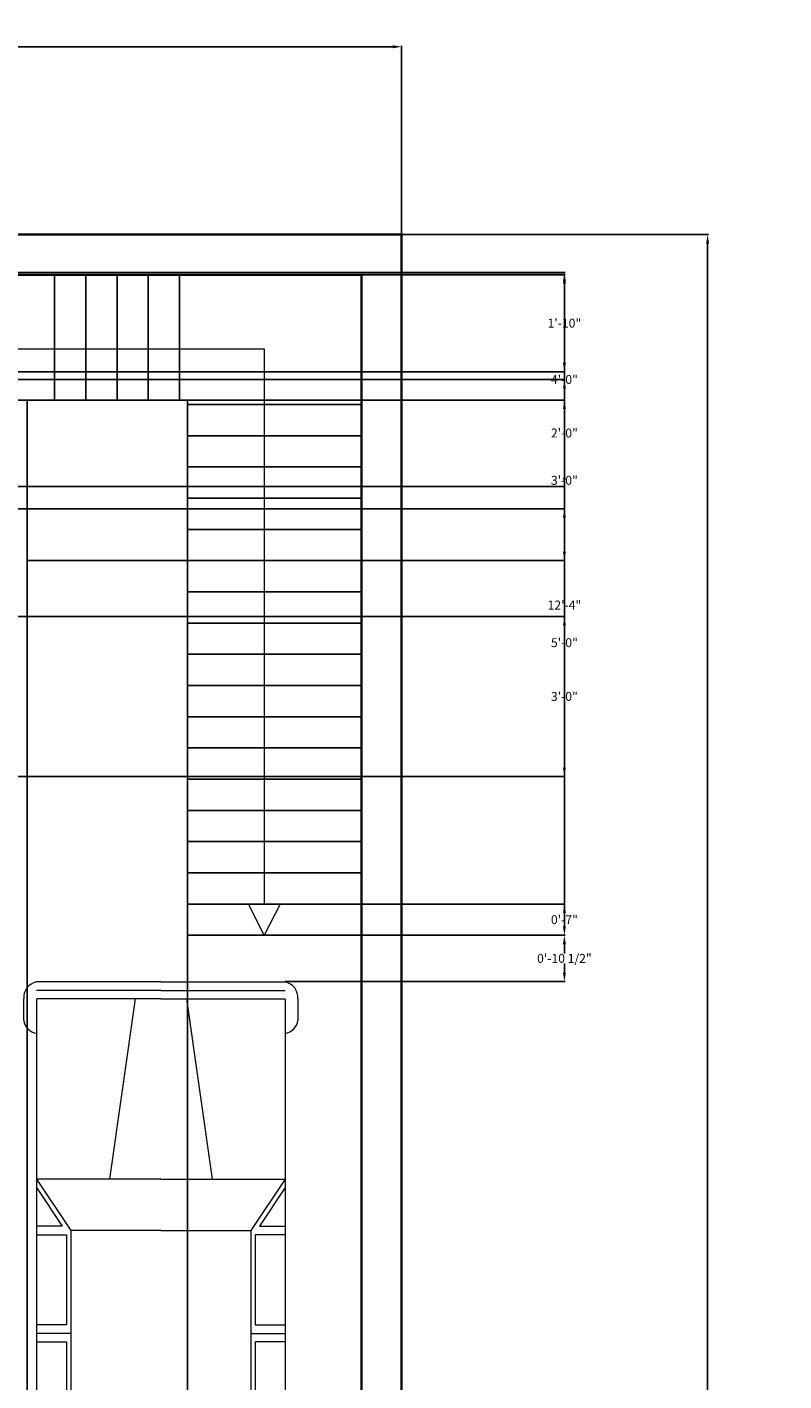
# Model space of a CAD drawing. Units: inches. Extents: x -83 to 408, y 158 to 919.
# Tile 5 of 5: x 238 to 408, y 586 to 889. Entities that reach past the tile are written whole.
import ezdxf

# ---------------------------------------------------------------- set-up
doc = ezdxf.new("R2010")
doc.units = ezdxf.units.IN
doc.header["$MEASUREMENT"] = 0
for name, color, linetype, lineweight in [('A-ANNO-DIMS', 2, 'Continuous', 18), ('A-ANNO-SYMB', 3, 'Continuous', 18), ('A-FLOR-STRS', 7, 'Continuous', 25), ('C-PKNG-VEHI', 8, 'Continuous', 18), ('L-WALL', 7, 'Continuous', 35)]:
    doc.layers.add(name, color=color, linetype=linetype, lineweight=lineweight)
doc.styles.get("Standard").update_dxf_attribs({"font": 'arial.ttf'})
doc.dimstyles.get("Standard").update_dxf_attribs({"dimtxt": 2, "dimasz": 2, "dimexe": 0.18, "dimexo": 0.0625, "dimgap": 0.09, "dimtad": 0, "dimtih": 1, "dimtoh": 1, "dimdec": 0, "dimzin": 0, "dimdsep": 46, "dimlunit": 3, "dimtxsty": 'Standard', "dimcen": 0.09, "dimadec": 0, "dimazin": 0, "dimtfac": 1, "dimtdec": 0, "dimtofl": 0, "dimtmove": 0, "dimatfit": 3, "dimfxl": 1, "dimtolj": 1, "dimtzin": 0, "dimarcsym": 0})

# ---------------------------------------------------------------- blocks, each defined once
blk = doc.blocks.new('*U15')
for p, q in [((5.44, 42.31), (12.12, 42.31)), ((189.69, 42.31), (183.01, 42.31)), ((0.1, -0.41), (0.1, 38.35)), ((2.77, -0.41), (2.77, 38.31)), ((5.44, -0.41), (5.44, 38.24)), ((5.45, 38.31), (16.12, 38.31)), ((16.12, 38.31), (180.34, 38.31)), ((61.52, -0.41), (61.52, 38.31)), ((61.52, 38.31), (77.54, 27.62)), ((64.19, 38.31), (76.2, 30.29)), ((76.2, 30.29), (76.2, 38.31)), ((78.87, 38.31), (78.87, 28.96)), ((106.91, 28.96), (106.91, 38.31)), ((109.58, 27.62), (109.58, 38.31)), ((112.25, 38.31), (112.25, 28.96)), ((140.29, 28.96), (140.29, 38.31)), ((141.62, 27.62), (149.64, 38.31)), ((149.64, -0.41), (149.64, 38.31)), ((189.69, 38.31), (179.01, 38.31)), ((189.69, -0.41), (189.69, 38.24)), ((192.36, -0.41), (192.36, 38.31)), ((195.03, -0.41), (195.03, 38.35)), ((77.54, 27.62), (141.62, 27.62)), ((77.54, -0.41), (77.54, 27.62)), ((78.87, 28.96), (106.91, 28.96)), ((112.25, 28.96), (140.29, 28.96)), ((141.62, -0.41), (141.62, 27.62)), ((5.44, 7.6), (61.52, 15.61)), ((0.1, -0.42), (0.1, -39.18)), ((2.77, -0.41), (2.77, -39.13)), ((5.44, -0.42), (5.44, -39.07)), ((61.52, -0.41), (61.52, -39.13)), ((77.54, -0.41), (77.54, -28.45)), ((141.62, -0.41), (141.62, -28.45)), ((149.64, -0.41), (149.64, -39.13)), ((189.69, -0.42), (189.69, -39.07)), ((192.36, -0.41), (192.36, -39.13)), ((195.03, -0.42), (195.03, -39.18)), ((5.44, -8.42), (61.52, -16.43)), ((61.52, -39.13), (77.54, -28.45)), ((77.54, -28.45), (141.62, -28.45)), ((109.58, -28.45), (109.58, -39.13)), ((141.62, -28.45), (149.64, -39.13)), ((64.19, -39.13), (76.2, -31.12)), ((76.2, -31.12), (76.2, -39.13)), ((78.87, -39.13), (78.87, -29.79)), ((78.87, -29.79), (106.91, -29.79)), ((106.91, -29.79), (106.91, -39.13)), ((112.25, -29.79), (140.29, -29.79)), ((112.25, -39.13), (112.25, -29.79)), ((140.29, -29.79), (140.29, -39.13)), ((5.45, -39.13), (16.12, -39.13)), ((16.12, -39.13), (180.34, -39.13)), ((189.69, -39.13), (179.01, -39.13)), ((5.44, -43.14), (12.12, -43.14)), ((189.69, -43.14), (183.01, -43.14))]:
    blk.add_line(p, q)
for centre, radius, start, end in [((5.06, 37.26), 5.06, 85.6455, 168.0943), ((11.45, 37.64), 4.72, 8.1301, 81.87), ((183.68, 37.64), 4.72, 98.13, 171.8699), ((190.07, 37.26), 5.06, 11.9057, 94.3545), ((5.06, -38.09), 5.06, 191.9057, 274.3545), ((11.45, -38.46), 4.72, 278.13, 351.8699), ((183.68, -38.46), 4.72, 188.1301, 261.87), ((190.07, -38.09), 5.06, 265.6455, 348.0943)]:
    blk.add_arc(centre, radius, start, end)
blk = doc.blocks.new('*D17')
at = {"layer": 'A-ANNO-DIMS', "color": 0, "lineweight": -2, "transparency": 16777216}
for p, q in [((322.25, 842.67), (390.98, 842.67)), ((390.8, 840.67), (390.8, 524.09)), ((390.8, 199.15), (390.8, 515.73)), ((322.25, 197.15), (390.98, 197.15))]:
    blk.add_line(p, q, dxfattribs=at)
at = {"layer": 'A-ANNO-DIMS', "color": 0, "transparency": 16777216}
for points in [[(390.47, 840.67), (391.14, 840.67), (390.8, 842.67)], [(390.47, 199.15), (391.14, 199.15), (390.8, 197.15)]]:
    blk.add_solid(points, dxfattribs=at)
at = {"layer": 'Defpoints', "color": 0, "transparency": 16777216}
for p in [(322.19, 842.67), (322.19, 197.15), (390.8, 197.15)]:
    blk.add_point(p, dxfattribs=at)
at = {"layer": 'A-ANNO-DIMS', "color": 0, "transparency": 16777216, "insert": (390.8, 519.91), "char_height": 2, "attachment_point": 5}
blk.add_mtext('\\A1;{\\H4x;53\'-10"}', dxfattribs=at)
blk = doc.blocks.new('*D18')
at = {"layer": 'A-ANNO-DIMS', "color": 0, "lineweight": -2, "transparency": 16777216}
for p, q in [((-40.81, 843.26), (-40.81, 884.97)), ((-38.81, 884.79), (126.86, 884.79)), ((320.19, 884.79), (154.52, 884.79)), ((322.19, 842.73), (322.19, 884.97))]:
    blk.add_line(p, q, dxfattribs=at)
at = {"layer": 'A-ANNO-DIMS', "color": 0, "transparency": 16777216}
for points in [[(-38.81, 885.12), (-38.81, 884.46), (-40.81, 884.79)], [(320.19, 885.12), (320.19, 884.46), (322.19, 884.79)]]:
    blk.add_solid(points, dxfattribs=at)
at = {"layer": 'Defpoints', "color": 0, "transparency": 16777216}
for p in [(322.19, 884.79), (-40.81, 843.2), (322.19, 842.67)]:
    blk.add_point(p, dxfattribs=at)
at = {"layer": 'A-ANNO-DIMS', "color": 0, "transparency": 16777216, "insert": (140.69, 884.79), "char_height": 2, "attachment_point": 5}
blk.add_mtext('\\A1;{\\H4x;30\'-3"}', dxfattribs=at)
blk = doc.blocks.new('*D48')
at = {"layer": 'A-ANNO-DIMS', "color": 0, "lineweight": -2, "transparency": 16777216}
for p, q in [((47.25, 834.2), (358.87, 834.2)), ((358.69, 832.2), (358.69, 811.31)), ((358.69, 788.2), (358.69, 809.09)), ((47.25, 786.2), (358.87, 786.2))]:
    blk.add_line(p, q, dxfattribs=at)
at = {"layer": 'A-ANNO-DIMS', "color": 0, "transparency": 16777216}
for points in [[(358.36, 832.2), (359.02, 832.2), (358.69, 834.2)], [(358.36, 788.2), (359.02, 788.2), (358.69, 786.2)]]:
    blk.add_solid(points, dxfattribs=at)
at = {"layer": 'Defpoints', "color": 0, "transparency": 16777216}
for p in [(47.19, 834.2), (47.19, 786.2), (358.69, 786.2)]:
    blk.add_point(p, dxfattribs=at)
at = {"layer": 'A-ANNO-DIMS', "color": 0, "transparency": 16777216, "insert": (358.69, 810.2), "char_height": 2, "attachment_point": 5}
blk.add_mtext('\\A1;4\'-0"', dxfattribs=at)
blk = doc.blocks.new('*D49')
at = {"layer": 'A-ANNO-DIMS', "color": 0, "lineweight": -2, "transparency": 16777216}
for p, q in [((47.25, 810.2), (358.87, 810.2)), ((358.69, 808.2), (358.69, 799.31)), ((358.69, 788.2), (358.69, 797.09)), ((47.25, 786.2), (358.87, 786.2))]:
    blk.add_line(p, q, dxfattribs=at)
at = {"layer": 'A-ANNO-DIMS', "color": 0, "transparency": 16777216}
for points in [[(358.36, 808.2), (359.02, 808.2), (358.69, 810.2)], [(358.36, 788.2), (359.02, 788.2), (358.69, 786.2)]]:
    blk.add_solid(points, dxfattribs=at)
at = {"layer": 'Defpoints', "color": 0, "transparency": 16777216}
for p in [(47.19, 810.2), (47.19, 786.2), (358.69, 786.2)]:
    blk.add_point(p, dxfattribs=at)
at = {"layer": 'A-ANNO-DIMS', "color": 0, "transparency": 16777216, "insert": (358.69, 798.2), "char_height": 2, "attachment_point": 5}
blk.add_mtext('\\A1;2\'-0"', dxfattribs=at)
blk = doc.blocks.new('*D50')
at = {"layer": 'A-ANNO-DIMS', "color": 0, "lineweight": -2, "transparency": 16777216}
for p, q in [((193.25, 757.08), (358.87, 757.08)), ((358.69, 755.08), (358.69, 740.25)), ((358.69, 723.2), (358.69, 738.03)), ((193.25, 721.2), (358.87, 721.2))]:
    blk.add_line(p, q, dxfattribs=at)
at = {"layer": 'A-ANNO-DIMS', "color": 0, "transparency": 16777216}
for points in [[(358.36, 755.08), (359.02, 755.08), (358.69, 757.08)], [(358.36, 723.2), (359.02, 723.2), (358.69, 721.2)]]:
    blk.add_solid(points, dxfattribs=at)
at = {"layer": 'Defpoints', "color": 0, "transparency": 16777216}
for p in [(193.19, 757.08), (193.19, 721.2), (358.69, 721.2)]:
    blk.add_point(p, dxfattribs=at)
at = {"layer": 'A-ANNO-DIMS', "color": 0, "transparency": 16777216, "insert": (358.69, 739.14), "char_height": 2, "attachment_point": 5}
blk.add_mtext('\\A1;3\'-0"', dxfattribs=at)
blk = doc.blocks.new('*D54')
at = {"layer": 'A-ANNO-DIMS', "color": 0, "lineweight": -2, "transparency": 16777216}
for p, q in [((193.25, 833.7), (358.87, 833.7)), ((358.69, 831.7), (358.69, 823.94)), ((358.69, 813.95), (358.69, 821.71)), ((193.25, 811.95), (358.87, 811.95))]:
    blk.add_line(p, q, dxfattribs=at)
at = {"layer": 'A-ANNO-DIMS', "color": 0, "transparency": 16777216}
for points in [[(358.36, 831.7), (359.02, 831.7), (358.69, 833.7)], [(358.36, 813.95), (359.02, 813.95), (358.69, 811.95)]]:
    blk.add_solid(points, dxfattribs=at)
at = {"layer": 'Defpoints', "color": 0, "transparency": 16777216}
for p in [(193.19, 833.7), (193.19, 811.95), (358.69, 811.95)]:
    blk.add_point(p, dxfattribs=at)
at = {"layer": 'A-ANNO-DIMS', "color": 0, "transparency": 16777216, "insert": (358.69, 822.83), "char_height": 2, "attachment_point": 5}
blk.add_mtext('\\A1;1\'-10"', dxfattribs=at)
blk = doc.blocks.new('*D56')
at = {"layer": 'A-ANNO-DIMS', "color": 0, "lineweight": -2, "transparency": 16777216}
for p, q in [((52.25, 781.2), (358.87, 781.2)), ((358.69, 779.2), (358.69, 752.31)), ((358.69, 723.2), (358.69, 750.09)), ((47.25, 721.2), (358.87, 721.2))]:
    blk.add_line(p, q, dxfattribs=at)
at = {"layer": 'A-ANNO-DIMS', "color": 0, "transparency": 16777216}
for points in [[(358.36, 779.2), (359.02, 779.2), (358.69, 781.2)], [(358.36, 723.2), (359.02, 723.2), (358.69, 721.2)]]:
    blk.add_solid(points, dxfattribs=at)
at = {"layer": 'Defpoints', "color": 0, "transparency": 16777216}
for p in [(52.19, 781.2), (47.19, 721.2), (358.69, 721.2)]:
    blk.add_point(p, dxfattribs=at)
at = {"layer": 'A-ANNO-DIMS', "color": 0, "transparency": 16777216, "insert": (358.69, 751.2), "char_height": 2, "attachment_point": 5}
blk.add_mtext('\\A1;5\'-0"', dxfattribs=at)
blk = doc.blocks.new('*D57')
at = {"layer": 'A-ANNO-DIMS', "color": 0, "lineweight": -2, "transparency": 16777216}
for p, q in [((274.19, 685.53), (274.19, 160.47)), ((313.19, 685.53), (313.19, 160.47)), ((276.19, 160.65), (290.94, 160.65)), ((311.19, 160.65), (296.44, 160.65))]:
    blk.add_line(p, q, dxfattribs=at)
at = {"layer": 'A-ANNO-DIMS', "color": 0, "transparency": 16777216}
for points in [[(276.19, 160.98), (276.19, 160.32), (274.19, 160.65)], [(311.19, 160.98), (311.19, 160.32), (313.19, 160.65)]]:
    blk.add_solid(points, dxfattribs=at)
at = {"layer": 'Defpoints', "color": 0, "transparency": 16777216}
for p in [(274.19, 685.59), (313.19, 685.59), (313.19, 160.65)]:
    blk.add_point(p, dxfattribs=at)
at = {"layer": 'A-ANNO-DIMS', "color": 0, "transparency": 16777216, "insert": (293.69, 160.65), "char_height": 2, "attachment_point": 5}
blk.add_mtext('\\A1;3\'-3"', dxfattribs=at)
blk = doc.blocks.new('*D58')
at = {"layer": 'A-ANNO-DIMS', "color": 0, "lineweight": -2, "transparency": 16777216}
for p, q in [((313.25, 833.67), (358.87, 833.67)), ((358.69, 831.67), (358.69, 760.72)), ((358.69, 687.59), (358.69, 758.54)), ((313.25, 685.59), (358.87, 685.59))]:
    blk.add_line(p, q, dxfattribs=at)
at = {"layer": 'A-ANNO-DIMS', "color": 0, "transparency": 16777216}
for points in [[(358.36, 831.67), (359.02, 831.67), (358.69, 833.67)], [(358.36, 687.59), (359.02, 687.59), (358.69, 685.59)]]:
    blk.add_solid(points, dxfattribs=at)
at = {"layer": 'Defpoints', "color": 0, "transparency": 16777216}
for p in [(313.19, 833.67), (358.69, 833.67), (313.19, 685.59)]:
    blk.add_point(p, dxfattribs=at)
at = {"layer": 'A-ANNO-DIMS', "color": 0, "transparency": 16777216, "insert": (358.69, 759.63), "char_height": 2, "attachment_point": 5}
blk.add_mtext('\\A1;12\'-4"', dxfattribs=at)
blk = doc.blocks.new('*D59')
at = {"layer": 'A-ANNO-DIMS', "color": 0, "lineweight": -2, "transparency": 16777216}
for p, q in [((202.19, 769.53), (202.19, 160.47)), ((238.19, 769.53), (238.19, 160.47)), ((204.19, 160.65), (217.44, 160.65)), ((236.19, 160.65), (222.94, 160.65))]:
    blk.add_line(p, q, dxfattribs=at)
at = {"layer": 'A-ANNO-DIMS', "color": 0, "transparency": 16777216}
for points in [[(204.19, 160.98), (204.19, 160.32), (202.19, 160.65)], [(236.19, 160.98), (236.19, 160.32), (238.19, 160.65)]]:
    blk.add_solid(points, dxfattribs=at)
at = {"layer": 'Defpoints', "color": 0, "transparency": 16777216}
for p in [(202.19, 769.59), (238.19, 769.59), (238.19, 160.65)]:
    blk.add_point(p, dxfattribs=at)
at = {"layer": 'A-ANNO-DIMS', "color": 0, "transparency": 16777216, "insert": (220.19, 160.65), "char_height": 2, "attachment_point": 5}
blk.add_mtext('\\A1;3\'-0"', dxfattribs=at)
blk = doc.blocks.new('*D60')
at = {"layer": 'A-ANNO-DIMS', "color": 0, "lineweight": -2, "transparency": 16777216}
for p, q in [((238.19, 805.53), (238.19, 160.47)), ((274.19, 805.53), (274.19, 160.47)), ((240.19, 160.65), (253.44, 160.65)), ((272.19, 160.65), (258.94, 160.65))]:
    blk.add_line(p, q, dxfattribs=at)
at = {"layer": 'A-ANNO-DIMS', "color": 0, "transparency": 16777216}
for points in [[(240.19, 160.98), (240.19, 160.32), (238.19, 160.65)], [(272.19, 160.98), (272.19, 160.32), (274.19, 160.65)]]:
    blk.add_solid(points, dxfattribs=at)
at = {"layer": 'Defpoints', "color": 0, "transparency": 16777216}
for p in [(238.19, 805.59), (274.19, 805.59), (274.19, 160.65)]:
    blk.add_point(p, dxfattribs=at)
at = {"layer": 'A-ANNO-DIMS', "color": 0, "transparency": 16777216, "insert": (256.19, 160.65), "char_height": 2, "attachment_point": 5}
blk.add_mtext('\\A1;3\'-0"', dxfattribs=at)
blk = doc.blocks.new('*D61')
at = {"layer": 'A-ANNO-DIMS', "color": 0, "lineweight": -2, "transparency": 16777216}
for p, q in [((238.25, 805.59), (358.87, 805.59)), ((358.69, 803.59), (358.69, 788.71)), ((358.69, 771.59), (358.69, 786.48)), ((238.25, 769.59), (358.87, 769.59))]:
    blk.add_line(p, q, dxfattribs=at)
at = {"layer": 'A-ANNO-DIMS', "color": 0, "transparency": 16777216}
for points in [[(358.36, 803.59), (359.02, 803.59), (358.69, 805.59)], [(358.36, 771.59), (359.02, 771.59), (358.69, 769.59)]]:
    blk.add_solid(points, dxfattribs=at)
at = {"layer": 'Defpoints', "color": 0, "transparency": 16777216}
for p in [(238.19, 805.59), (358.69, 805.59), (238.19, 769.59)]:
    blk.add_point(p, dxfattribs=at)
at = {"layer": 'A-ANNO-DIMS', "color": 0, "transparency": 16777216, "insert": (358.69, 787.59), "char_height": 2, "attachment_point": 5}
blk.add_mtext('\\A1;3\'-0"', dxfattribs=at)
blk = doc.blocks.new('*D62')
at = {"layer": 'A-ANNO-DIMS', "color": 0, "lineweight": -2, "transparency": 16777216}
for p, q in [((272.31, 833.67), (-77.49, 833.67)), ((-77.31, 831.67), (-77.31, 820.72)), ((-77.31, 807.59), (-77.31, 818.54)), ((274.13, 805.59), (-77.49, 805.59))]:
    blk.add_line(p, q, dxfattribs=at)
at = {"layer": 'A-ANNO-DIMS', "color": 0, "transparency": 16777216}
for points in [[(-77.64, 831.67), (-76.98, 831.67), (-77.31, 833.67)], [(-77.64, 807.59), (-76.98, 807.59), (-77.31, 805.59)]]:
    blk.add_solid(points, dxfattribs=at)
at = {"layer": 'Defpoints', "color": 0, "transparency": 16777216}
for p in [(-77.31, 833.67), (272.37, 833.67), (274.19, 805.59)]:
    blk.add_point(p, dxfattribs=at)
at = {"layer": 'A-ANNO-DIMS', "color": 0, "transparency": 16777216, "insert": (-77.31, 819.63), "char_height": 2, "attachment_point": 5}
blk.add_mtext('\\A1;2\'-4"', dxfattribs=at)
blk = doc.blocks.new('*D63')
at = {"layer": 'A-ANNO-DIMS', "color": 0, "lineweight": -2, "transparency": 16777216}
for p, q in [((313.25, 692.59), (358.87, 692.59)), ((358.69, 690.59), (358.69, 690.2)), ((358.69, 687.59), (358.69, 687.98)), ((313.25, 685.59), (358.87, 685.59))]:
    blk.add_line(p, q, dxfattribs=at)
at = {"layer": 'A-ANNO-DIMS', "color": 0, "transparency": 16777216}
for points in [[(358.36, 690.59), (359.02, 690.59), (358.69, 692.59)], [(358.36, 687.59), (359.02, 687.59), (358.69, 685.59)]]:
    blk.add_solid(points, dxfattribs=at)
at = {"layer": 'Defpoints', "color": 0, "transparency": 16777216}
for p in [(313.19, 692.59), (358.69, 692.59), (313.19, 685.59)]:
    blk.add_point(p, dxfattribs=at)
at = {"layer": 'A-ANNO-DIMS', "color": 0, "transparency": 16777216, "insert": (358.69, 689.09), "char_height": 2, "attachment_point": 5}
blk.add_mtext('\\A1;0\'-7"', dxfattribs=at)
blk = doc.blocks.new('*D70')
at = {"layer": 'A-ANNO-DIMS', "color": 0, "lineweight": -2, "transparency": 16777216}
for p, q in [((313.25, 685.59), (358.87, 685.59)), ((358.69, 683.59), (358.69, 681.54)), ((358.69, 677.24), (358.69, 679.29)), ((296.03, 675.24), (358.87, 675.24))]:
    blk.add_line(p, q, dxfattribs=at)
at = {"layer": 'A-ANNO-DIMS', "color": 0, "transparency": 16777216}
for points in [[(358.36, 683.59), (359.02, 683.59), (358.69, 685.59)], [(358.36, 677.24), (359.02, 677.24), (358.69, 675.24)]]:
    blk.add_solid(points, dxfattribs=at)
at = {"layer": 'Defpoints', "color": 0, "transparency": 16777216}
for p in [(313.19, 685.59), (358.69, 685.59), (295.97, 675.24)]:
    blk.add_point(p, dxfattribs=at)
at = {"layer": 'A-ANNO-DIMS', "color": 0, "transparency": 16777216, "insert": (358.69, 680.42), "char_height": 2, "attachment_point": 5}
blk.add_mtext('\\A1;0\'-10 1/2"', dxfattribs=at)

msp = doc.modelspace()

# ---------------------------------------------------------------- linework, layer by layer
at = {"layer": 'A-ANNO-SYMB'}
for p, q in [((220.19, 817.05), (291.39, 817.05)), ((291.39, 817.05), (291.39, 692.59))]:
    msp.add_line(p, q, dxfattribs=at)
msp.add_lwpolyline([(291.39, 685.59), (287.81, 692.59), (294.97, 692.59)], close=True, dxfattribs=at)
at = {"layer": 'A-FLOR-STRS'}
for p, q in [((244.37, 805.59), (244.37, 833.67)), ((251.37, 805.59), (251.37, 833.67)), ((258.37, 805.59), (258.37, 833.67)), ((265.37, 805.59), (265.37, 833.67)), ((272.37, 805.59), (272.37, 833.67)), ((238.19, 805.59), (274.19, 805.59)), ((274.19, 805.59), (274.19, 685.59)), ((274.19, 804.59), (313.19, 804.59)), ((274.19, 797.59), (313.19, 797.59)), ((274.19, 790.59), (313.19, 790.59)), ((274.19, 783.59), (313.19, 783.59)), ((274.19, 776.59), (313.19, 776.59)), ((274.19, 769.59), (313.19, 769.59)), ((274.19, 762.59), (313.19, 762.59)), ((274.19, 755.59), (313.19, 755.59)), ((274.19, 748.59), (313.19, 748.59)), ((274.19, 741.59), (313.19, 741.59)), ((274.19, 734.59), (313.19, 734.59)), ((274.19, 727.59), (313.19, 727.59)), ((274.19, 720.59), (313.19, 720.59)), ((274.19, 713.59), (313.19, 713.59)), ((274.19, 706.59), (313.19, 706.59)), ((274.19, 699.59), (313.19, 699.59)), ((274.19, 692.59), (313.19, 692.59)), ((274.19, 685.59), (313.19, 685.59))]:
    msp.add_line(p, q, dxfattribs=at)
at = {"layer": 'L-WALL'}
for p, q in [((322.19, 842.67), (202.19, 842.67)), ((322.19, 842.67), (322.19, 197.15)), ((202.19, 833.67), (313.19, 833.67)), ((313.19, 833.67), (313.19, 197.15))]:
    msp.add_line(p, q, dxfattribs=at)

# ---------------------------------------------------------------- block references
at = {"layer": 'C-PKNG-VEHI', "xscale": 0.7198545955529133, "yscale": 0.7198545955529133, "zscale": 0.7198545955529133, "rotation": 270}
msp.add_blockref('*U15', (268.48, 675.24), dxfattribs=at)

# ---------------------------------------------------------------- dimensions: what is measured, and where the dimension line sits
at = {"layer": 'A-ANNO-DIMS'}
dim = msp.add_linear_dim(base=(322.19, 884.79), p1=(-40.81, 843.2), p2=(322.19, 842.67), text='{\\H4x;<>}', dimstyle='Standard', override={"dimclrd": 0, "dimclre": 0, "dimclrt": 0}, dxfattribs=at)
dim.commit()
dim.dimension.update_dxf_attribs({"geometry": '*D18', "text_midpoint": (140.69, 884.79)})
dim = msp.add_linear_dim(base=(390.8, 197.15), p1=(322.19, 842.67), p2=(322.19, 197.15), angle=90, text='{\\H4x;<>}', dimstyle='Standard', override={"dimclrd": 0, "dimclre": 0, "dimclrt": 0}, dxfattribs=at)
dim.commit()
dim.dimension.update_dxf_attribs({"geometry": '*D17', "text_midpoint": (390.8, 519.91)})
for base, p1, p2, picture, middle in [((-77.31, 833.67), (274.19, 805.59), (272.37, 833.67), '*D62', (-77.31, 819.63)), ((358.69, 786.2), (47.19, 834.2), (47.19, 786.2), '*D48', (358.69, 810.2)), ((358.6891, 811.95026), (193.1891, 833.70029), (193.1891, 811.95026), '*D54', (358.6891, 822.82528)), ((358.69, 833.67), (313.19, 685.59), (313.19, 833.67), '*D58', (358.69, 759.63)), ((358.69, 786.2), (47.19, 810.2), (47.19, 786.2), '*D49', (358.69, 798.2)), ((358.69, 805.59), (238.19, 769.59), (238.19, 805.59), '*D61', (358.69, 787.59)), ((358.69, 721.2), (52.19, 781.2), (47.19, 721.2), '*D56', (358.69, 751.2)), ((358.69, 721.2), (193.19, 757.08), (193.19, 721.2), '*D50', (358.69, 739.14)), ((358.69, 692.59), (313.19, 685.59), (313.19, 692.59), '*D63', (358.69, 689.09)), ((358.6891, 685.5933), (295.9713, 675.2383), (313.1891, 685.5933), '*D70', (358.6891, 680.4158))]:
    dim = msp.add_linear_dim(base=base, p1=p1, p2=p2, angle=90, dimstyle='Standard', override={"dimdec": 1, "dimlfac": 1, "dimrnd": 0, "dimzin": 1, "dimdsep": 46, "dimlunit": 4, "dimfrac": 2}, dxfattribs=at)
    dim.commit()
    dim.dimension.update_dxf_attribs({"geometry": picture, "text_midpoint": middle})
for base, p1, p2, picture, middle in [((274.19, 160.65), (238.19, 805.59), (274.19, 805.59), '*D60', (256.19, 160.65)), ((238.19, 160.65), (202.19, 769.59), (238.19, 769.59), '*D59', (220.19, 160.65)), ((313.19, 160.65), (274.19, 685.59), (313.19, 685.59), '*D57', (293.69, 160.65))]:
    dim = msp.add_linear_dim(base=base, p1=p1, p2=p2, dimstyle='Standard', override={"dimdec": 1, "dimlfac": 1, "dimrnd": 0, "dimzin": 1, "dimdsep": 46, "dimlunit": 4, "dimfrac": 2}, dxfattribs=at)
    dim.commit()
    dim.dimension.update_dxf_attribs({"geometry": picture, "text_midpoint": middle})

doc.saveas('drawing.dxf')
